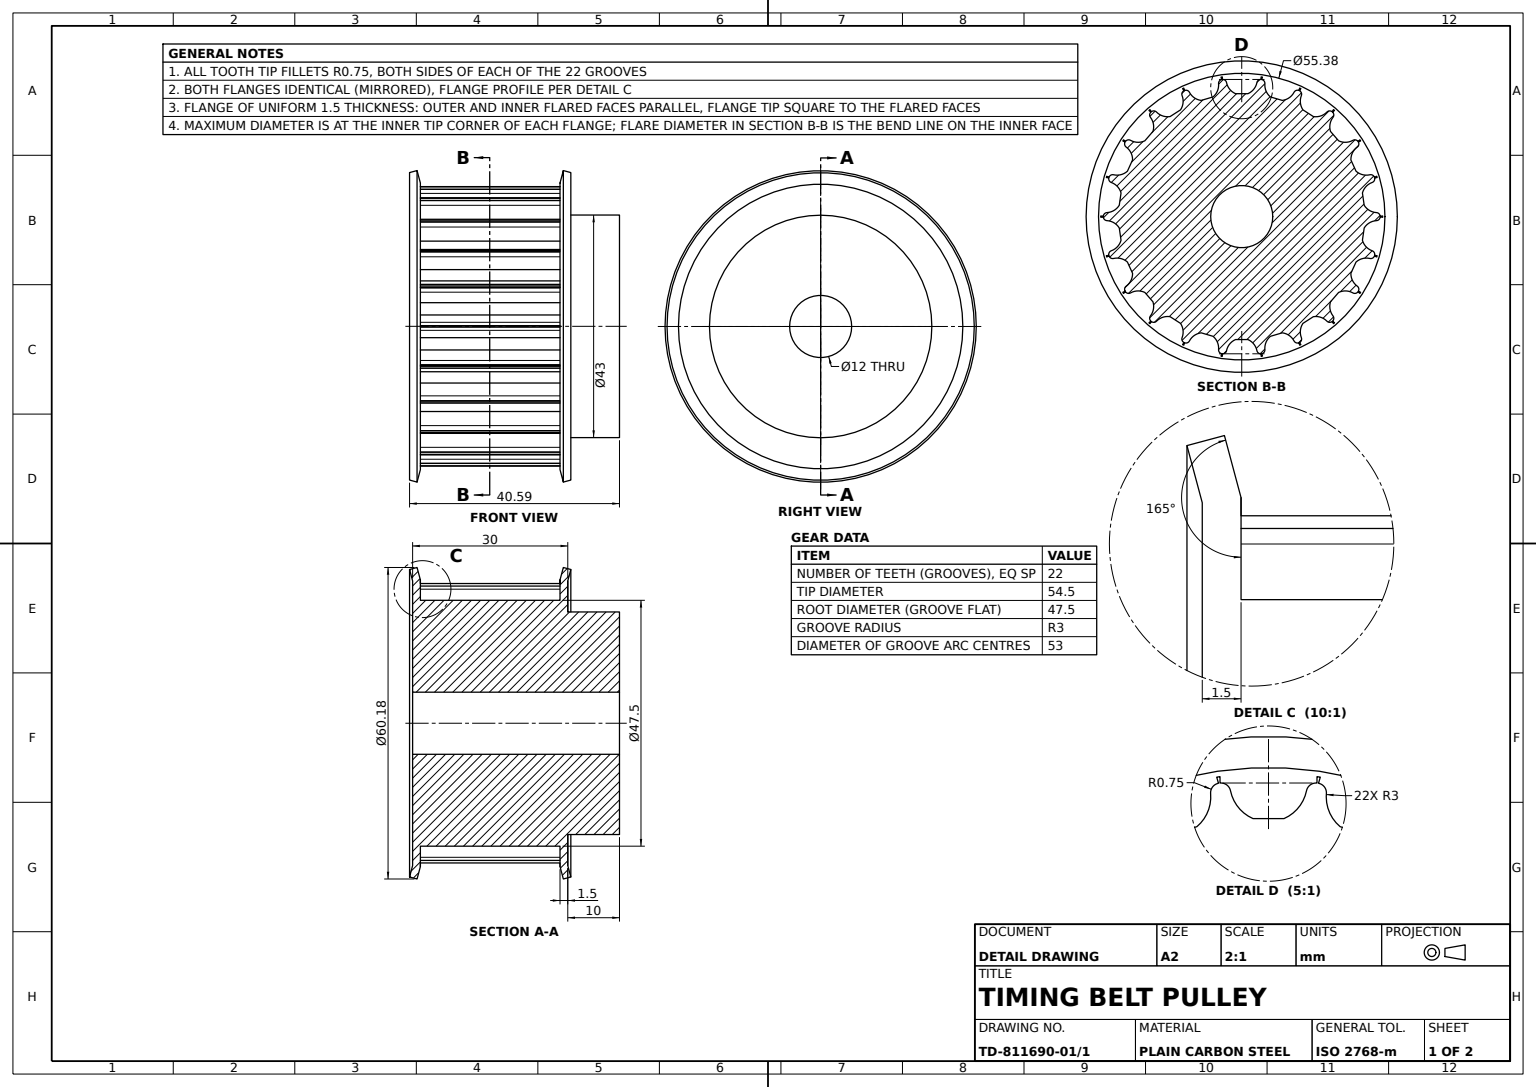
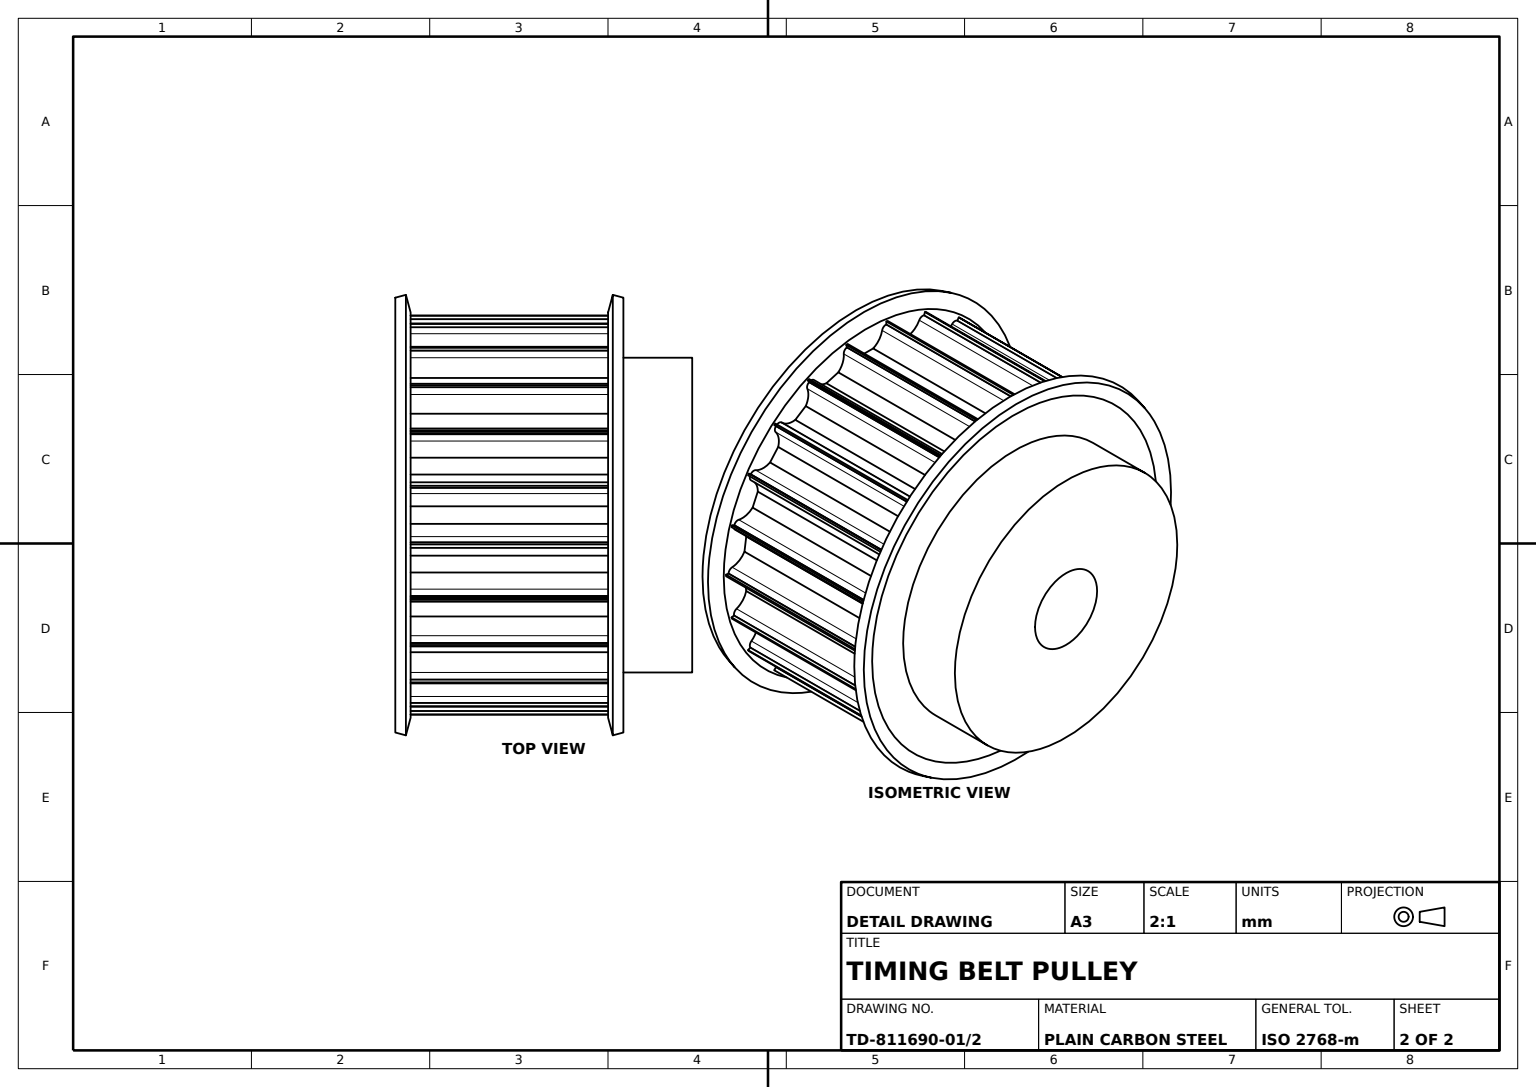
SolidWorks part; units mm, degrees
material "Plain Carbon Steel"
ref_plane "Front Plane" through (0, 0, 0) normal (0, 0, 1) x (1, 0, 0)
ref_plane "Top Plane" through (0, 0, 0) normal (0, 1, 0) x (1, 0, 0)
ref_plane "Right Plane" through (0, 0, 0) normal (1, 0, 0) x (0, 0, -1)
ref_axis "Wheel Axis" through (0, 0, -42.0296) along (0, 0, 1)
sketch "Wheel Body Profile" plane through (0, 0, 0) normal (1, 0, 0) x (0, 0, -1)
  line L0 (0, 6) -> (0, 27.25)
  line L1 (0, 27.25) -> (30, 27.25)
  line L2 (30, 27.25) -> (30, 21.5)
  line L3 (30, 21.5) -> (40, 21.5)
  line L4 (40, 21.5) -> (40, 6)
  line L5 (40, 6) -> (0, 6)
  line L6 (42.0296, 0) -> (-2.6216, 0) construction
  dimension "D1" = 6
  dimension "D2" = 21.25
  dimension "D3" = 30
  dimension "D4" = 10
  dimension "D5" = 15.5
revolve "Wheel Body" add sketch "Wheel Body Profile" angle 360 about axis through (0, 0, -42.0296) along (0, 0, 1)
sketch "Tooth Groove Profile" plane through (0, 0, 0) normal (0, 0, 1) x (1, 0, 0)
  line L0 (3.6742, 26.5) -> (3.75, 26.5)
  line L1 (-3.75, 28.5) -> (3.75, 28.5)
  line L2 (-3.75, 28.5) -> (-3.75, 26.5)
  line L3 (-3.75, 26.5) -> (-3.6742, 26.5)
  line L4 (3.75, 28.5) -> (3.75, 26.5)
  line L5 (-1.199, 23.75) -> (1.199, 23.75)
  arc A0 (-2.9394, 25.9) -> (-1.199, 23.75) centre (0, 26.5) ccw
  arc A1 (-2.9394, 25.9) -> (-3.6742, 26.5) centre (-3.6742, 25.75) ccw
  arc A2 (2.9394, 25.9) -> (3.6742, 26.5) centre (3.6742, 25.75) cw
  arc A3 (1.199, 23.75) -> (2.9394, 25.9) centre (0, 26.5) ccw
  point P13 (-3, 26.5)
  point P16 (3, 26.5)
  dimension "D3" = 3
  dimension "D5" = 0.75
  dimension "D1" = 7.5
  dimension "D2" = 2
  dimension "D4" = 26.5
  dimension "D6" = 2.75
extrude "Tooth Groove Cut" cut sketch "Tooth Groove Profile" against normal through all
pattern_circular "Tooth Groove Pattern 22x" count 22 over 360 about axis through (0, 0, 0) along (0, 0, 1) of "Tooth Groove Cut"
sketch "Flange Profile" plane through (0, 0, 0) normal (1, 0, 0) x (0, 0, -1)
  line L0 (0, 25.679) -> (0, 23.1257) construction
  line L1 (0, 22.6907) -> (1.5, 22.6907)
  line L2 (0, 22.6907) -> (0, 27.6907)
  line L3 (0, 27.6907) -> (1.5, 27.6907) construction
  line L4 (1.5, 22.6907) -> (1.5, 27.6907)
  line L5 (1.5, 27.6907) -> (0.0511, 27.3025) construction
  line L6 (1.5, 27.6907) -> (0.8569, 30.0907)
  line L7 (0.0511, 27.3025) -> (-0.592, 29.7025)
  line L8 (0.8569, 30.0907) -> (-0.592, 29.7025)
  line L9 (0, 26.9907) -> (30, 26.9907) construction
  line L10 (15, 26.9907) -> (15, -26.9907) construction
  line L11 (30, -26.9907) -> (0, -26.9907) construction
  line L12 (28.5, 27.6907) -> (29.9489, 27.3025) construction
  line L13 (30, 27.6907) -> (28.5, 27.6907) construction
  line L14 (29.1431, 30.0907) -> (30.592, 29.7025)
  line L15 (29.9489, 27.3025) -> (30.592, 29.7025)
  line L16 (28.5, 27.6907) -> (29.1431, 30.0907)
  line L17 (28.5, 22.6907) -> (28.5, 27.6907)
  line L18 (30, 22.6907) -> (30, 27.6907)
  line L19 (30, 22.6907) -> (28.5, 22.6907)
  dimension "D1" = 1.5
  dimension "D2" = 5
  dimension "D3" = 2.4
  dimension "D4" = 1.5
  dimension "D5" = 165
  dimension "D6" = 0.7
revolve "Belt Flanges" add sketch "Flange Profile" angle 360 about axis through (0, 0, -42.0296) along (0, 0, 1)
